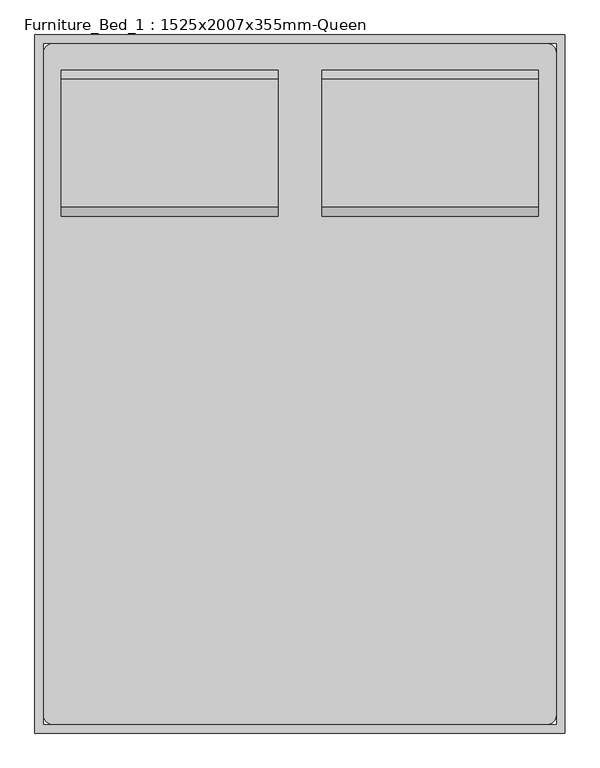
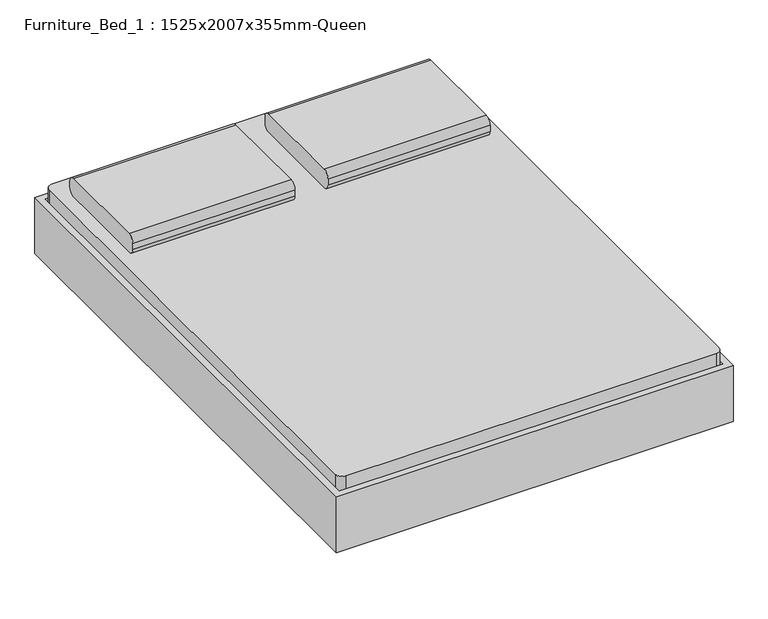
"""IFC4 building model written with IfcOpenShell, lengths in millimetres: furniture geometry, Furniture_Bed_1 : 1525x2007x355mm-Queen."""

from ifc_helpers import new_model, si_unit, point, frame, frame_2d, origin, place, context, project, spatial, polyline, circle_curve, trimmed, segment, composite_curve, outline, extrude, source, transform, mapped, element, save
from ifc_brep_helpers import plane_surface, cylinder_surface, revolved_surface, advanced_brep


def furniture_bed_1_1525x2007x355mm_queen_b7403446(model_context):
    return source(origin(), model_context, "Body", "SolidModel", [
        advanced_brep(
        [(-397.947541, -933.1295082, 196.85), (-397.947541, -933.1295082, 177.8), (-397.947541, -1009.3295082, 177.8), (-397.947541, -1009.3295082, 196.85), (-335.0113525, -933.1295082, 196.85), (-347.147541, -933.1295082, 177.8), (-347.147541, -1009.3295082, 177.8), (-335.0113525, -1009.3295082, 196.85), (-253.8115092, -933.1295082, 22.716374), (-271.0766725, -933.1295082, 14.6654962), (-271.0766725, -1009.3295082, 14.6654962), (-253.8115092, -1009.3295082, 22.716374), (-248.0564547, -933.1295082, 0.0), (-248.0564547, -933.1295082, 19.05), (-248.0564547, -1009.3295082, 0.0), (-248.0564547, -1009.3295082, 19.05), (-169.4439489, -933.1295082, 19.05), (-169.4439489, -933.1295082, 0.0), (-169.4439489, -1009.3295082, 0.0), (-169.4439489, -1009.3295082, 19.05), (-156.7439489, -933.1295082, 3.4029547), (-166.2689489, -933.1295082, 19.9007387), (-156.7439489, -1009.3295082, 3.4029547), (-166.2689489, -1009.3295082, 19.9007387), (-101.7513357, -933.1295082, 57.15), (-96.6469036, -933.1295082, 38.1), (-96.6469036, -1009.3295082, 38.1), (-101.7513357, -1009.3295082, 57.15), (780.0562537, -933.1295082, 57.15), (774.9518216, -933.1295082, 38.1), (774.9518216, -1009.3295082, 38.1), (780.0562537, -1009.3295082, 57.15), (844.5738669, -933.1295082, 19.9007387), (835.0488669, -933.1295082, 3.4029547), (835.0488669, -1009.3295082, 3.4029547), (844.5738669, -1009.3295082, 19.9007387), (847.7488669, -933.1295082, 0.0), (847.7488669, -933.1295082, 19.05), (847.7488669, -1009.3295082, 0.0), (847.7488669, -1009.3295082, 19.05), (926.3613728, -933.1295082, 19.05), (926.3613728, -933.1295082, 0.0), (926.3613728, -1009.3295082, 0.0), (926.3613728, -1009.3295082, 19.05), (949.3815906, -933.1295082, 14.6654962), (932.1164272, -933.1295082, 22.716374), (949.3815906, -1009.3295082, 14.6654962), (932.1164272, -1009.3295082, 22.716374), (1013.3162705, -933.1295082, 196.85), (1025.452459, -933.1295082, 177.8), (1025.452459, -1009.3295082, 177.8), (1013.3162705, -1009.3295082, 196.85), (1076.252459, -933.1295082, 196.85), (1076.252459, -1009.3295082, 196.85), (1076.252459, -1009.3295082, 177.8), (1076.252459, -933.1295082, 177.8)],
        [
            (0, 1),
            (1, 2),
            (2, 3),
            (3, 0),
            (0, 4),
            (4, 5),
            (5, 1),
            (5, 6),
            (6, 2),
            (6, 7),
            (7, 3),
            (7, 4),
            (4, 8),
            (8, 9),
            (9, 5),
            (9, 10),
            (10, 6),
            (10, 11),
            (11, 7),
            (11, 8),
            (12, 9, circle_curve(frame((-248.0564547, -933.1295082, 25.4), z_axis=(0.0, 1.0, 0.0), x_axis=(-0.9063077870366627, 0.0, -0.42261826174067213)), 25.4)),
            (8, 13, circle_curve(frame((-248.0564547, -933.1295082, 25.4), z_axis=(0.0, -1.0, 0.0), x_axis=(-0.9063077870366627, 0.0, -0.42261826174067213)), 6.35)),
            (13, 12),
            (14, 10, circle_curve(frame((-248.0564547, -1009.3295082, 25.4), z_axis=(0.0, 1.0, 0.0), x_axis=(-0.9063077870366627, 0.0, -0.42261826174067213)), 25.4)),
            (12, 14),
            (15, 11, circle_curve(frame((-248.0564547, -1009.3295082, 25.4), z_axis=(0.0, 1.0, 0.0), x_axis=(-0.9063077870366627, 0.0, -0.42261826174067213)), 6.35)),
            (14, 15),
            (15, 13),
            (13, 16),
            (16, 17),
            (17, 12),
            (17, 18),
            (18, 14),
            (18, 19),
            (19, 15),
            (19, 16),
            (20, 17, circle_curve(frame((-169.4439489, -933.1295082, 25.4), z_axis=(0.0, 1.0, 0.0), x_axis=(0.0, 0.0, -1.0)), 25.4)),
            (16, 21, circle_curve(frame((-169.4439489, -933.1295082, 25.4), z_axis=(0.0, -1.0, 0.0), x_axis=(0.0, 0.0, -1.0)), 6.35)),
            (21, 20),
            (22, 18, circle_curve(frame((-169.4439489, -1009.3295082, 25.4), z_axis=(0.0, 1.0, 0.0), x_axis=(0.0, 0.0, -1.0)), 25.4)),
            (20, 22),
            (23, 19, circle_curve(frame((-169.4439489, -1009.3295082, 25.4), z_axis=(0.0, 1.0, 0.0), x_axis=(0.0, 0.0, -1.0)), 6.35)),
            (22, 23),
            (23, 21),
            (21, 24),
            (24, 25),
            (25, 20),
            (25, 26),
            (26, 22),
            (26, 27),
            (27, 23),
            (27, 24),
            (24, 28),
            (28, 29),
            (29, 25),
            (29, 30),
            (30, 26),
            (30, 31),
            (31, 27),
            (31, 28),
            (28, 32),
            (32, 33),
            (33, 29),
            (33, 34),
            (34, 30),
            (34, 35),
            (35, 31),
            (35, 32),
            (36, 33, circle_curve(frame((847.7488669, -933.1295082, 25.4), z_axis=(0.0, 1.0, 0.0), x_axis=(-0.5000000000000486, 0.0, -0.8660254037844105)), 25.4)),
            (32, 37, circle_curve(frame((847.7488669, -933.1295082, 25.4), z_axis=(0.0, -1.0, 0.0), x_axis=(-0.5000000000000486, 0.0, -0.8660254037844105)), 6.35)),
            (37, 36),
            (38, 34, circle_curve(frame((847.7488669, -1009.3295082, 25.4), z_axis=(0.0, 1.0, 0.0), x_axis=(-0.5000000000000486, 0.0, -0.8660254037844105)), 25.4)),
            (36, 38),
            (39, 35, circle_curve(frame((847.7488669, -1009.3295082, 25.4), z_axis=(0.0, 1.0, 0.0), x_axis=(-0.5000000000000486, 0.0, -0.8660254037844105)), 6.35)),
            (38, 39),
            (39, 37),
            (37, 40),
            (40, 41),
            (41, 36),
            (41, 42),
            (42, 38),
            (42, 43),
            (43, 39),
            (43, 40),
            (44, 41, circle_curve(frame((926.3613728, -933.1295082, 25.4), z_axis=(0.0, 1.0, 0.0), x_axis=(0.0, 0.0, -1.0)), 25.4)),
            (40, 45, circle_curve(frame((926.3613728, -933.1295082, 25.4), z_axis=(0.0, -1.0, 0.0), x_axis=(0.0, 0.0, -1.0)), 6.35)),
            (45, 44),
            (46, 42, circle_curve(frame((926.3613728, -1009.3295082, 25.4), z_axis=(0.0, 1.0, 0.0), x_axis=(0.0, 0.0, -1.0)), 25.4)),
            (44, 46),
            (47, 43, circle_curve(frame((926.3613728, -1009.3295082, 25.4), z_axis=(0.0, 1.0, 0.0), x_axis=(0.0, 0.0, -1.0)), 6.35)),
            (46, 47),
            (47, 45),
            (45, 48),
            (48, 49),
            (49, 44),
            (49, 50),
            (50, 46),
            (50, 51),
            (51, 47),
            (51, 48),
            (52, 53),
            (53, 54),
            (54, 55),
            (55, 52),
            (48, 52),
            (55, 49),
            (54, 50),
            (53, 51),
        ],
        [
            plane_surface(frame((-397.947541, -1237.9295082, -127.5947323), z_axis=(-1.0, 0.0, 0.0), x_axis=(0.0, 1.0, 0.0))),
            plane_surface(frame((-397.947541, -933.1295082, 196.85), z_axis=(0.0, 1.0, 0.0), x_axis=(1.0, 0.0, 0.0))),
            plane_surface(frame((-397.947541, -933.1295082, 177.8), z_axis=(0.0, 0.0, -1.0), x_axis=(1.0, 0.0, 0.0))),
            plane_surface(frame((-397.947541, -1009.3295082, 177.8), z_axis=(0.0, -1.0, 0.0), x_axis=(1.0, 0.0, 0.0))),
            plane_surface(frame((-397.947541, -1009.3295082, 196.85), z_axis=(0.0, 0.0, 1.0), x_axis=(1.0, 0.0, 0.0))),
            plane_surface(frame((-335.0113525, -933.1295082, 196.85), z_axis=(0.0, 1.0000000000000002, 0.0), x_axis=(0.4226182617406718, 0.0, -0.9063077870366629))),
            plane_surface(frame((-347.147541, -933.1295082, 177.8), z_axis=(-0.906307787036663, 0.0, -0.4226182617406716), x_axis=(0.4226182617406716, 0.0, -0.906307787036663))),
            plane_surface(frame((-347.147541, -1009.3295082, 177.8), z_axis=(0.0, -1.0000000000000002, 0.0), x_axis=(0.4226182617406718, 0.0, -0.9063077870366629))),
            plane_surface(frame((-335.0113525, -1009.3295082, 196.85), z_axis=(0.9063077870366628, 0.0, 0.42261826174067196), x_axis=(0.42261826174067196, 0.0, -0.9063077870366628))),
            plane_surface(frame((-248.0564547, -933.1295082, 25.4), z_axis=(0.0, 1.0, 0.0), x_axis=(-0.9063077870366627, 0.0, -0.42261826174067213))),
            cylinder_surface(frame((-248.0564547, -1237.9295082, 25.4), z_axis=(0.0, -1.0, 0.0), x_axis=(-0.9063077870366627, 0.0, -0.42261826174067213)), 25.4),
            plane_surface(frame((-248.0564547, -1009.3295082, 25.4), z_axis=(0.0, -1.0, 0.0), x_axis=(-0.9063077870366627, 0.0, -0.42261826174067213))),
            revolved_surface(polyline([(-253.81150914768278, -1009.3295082, 22.716374037946732), (-253.81150914768278, -933.1295082, 22.716374037946732)]), (-248.0564547, -1237.9295082, 25.4), (0.0, -1.0, 0.0)),
            plane_surface(frame((-248.0564547, -933.1295082, 19.05), z_axis=(0.0, 1.0, 0.0), x_axis=(1.0, 0.0, 0.0))),
            plane_surface(frame((-248.0564547, -933.1295082, 0.0), z_axis=(0.0, 0.0, -1.0), x_axis=(1.0, 0.0, 0.0))),
            plane_surface(frame((-248.0564547, -1009.3295082, 0.0), z_axis=(0.0, -1.0, 0.0), x_axis=(1.0, 0.0, 0.0))),
            plane_surface(frame((-248.0564547, -1009.3295082, 19.05), z_axis=(0.0, 0.0, 1.0), x_axis=(1.0, 0.0, 0.0))),
            plane_surface(frame((-169.4439489, -933.1295082, 25.4), z_axis=(0.0, 1.0, 0.0), x_axis=(0.0, 0.0, -1.0))),
            cylinder_surface(frame((-169.4439489, -1237.9295082, 25.4), z_axis=(0.0, -1.0, 0.0), x_axis=(0.0, 0.0, -1.0)), 25.4),
            plane_surface(frame((-169.4439489, -1009.3295082, 25.4), z_axis=(0.0, -1.0, 0.0), x_axis=(0.0, 0.0, -1.0))),
            revolved_surface(polyline([(-169.4439489, -1009.3295082, 19.049999999999997), (-169.4439489, -933.1295082, 19.049999999999997)]), (-169.4439489, -1237.9295082, 25.4), (0.0, -1.0, 0.0)),
            plane_surface(frame((-166.2689489, -933.1295082, 19.9007387), z_axis=(0.0, 1.0, 0.0), x_axis=(0.8660254037844786, 0.0, 0.4999999999999309))),
            plane_surface(frame((-156.7439489, -933.1295082, 3.4029547), z_axis=(0.4999999999999315, 0.0, -0.8660254037844782), x_axis=(0.8660254037844782, 0.0, 0.4999999999999315))),
            plane_surface(frame((-156.7439489, -1009.3295082, 3.4029547), z_axis=(0.0, -1.0, 0.0), x_axis=(0.8660254037844788, 0.0, 0.49999999999993044))),
            plane_surface(frame((-166.2689489, -1009.3295082, 19.9007387), z_axis=(-0.4999999999999304, 0.0, 0.8660254037844789), x_axis=(0.8660254037844789, 0.0, 0.4999999999999304))),
            plane_surface(frame((-101.7513357, -933.1295082, 57.15), z_axis=(0.0, 1.0, 0.0), x_axis=(1.0, 0.0, 0.0))),
            plane_surface(frame((-96.6469036, -933.1295082, 38.1), z_axis=(0.0, 0.0, -1.0), x_axis=(1.0, 0.0, 0.0))),
            plane_surface(frame((-96.6469036, -1009.3295082, 38.1), z_axis=(0.0, -1.0, 0.0), x_axis=(1.0, 0.0, 0.0))),
            plane_surface(frame((-101.7513357, -1009.3295082, 57.15), z_axis=(0.0, 0.0, 1.0), x_axis=(1.0, 0.0, 0.0))),
            plane_surface(frame((780.0562537, -933.1295082, 57.15), z_axis=(0.0, 1.0, 0.0), x_axis=(0.866025403784412, 0.0, -0.5000000000000463))),
            plane_surface(frame((774.9518216, -933.1295082, 38.1), z_axis=(-0.500000000000047, 0.0, -0.8660254037844116), x_axis=(0.8660254037844116, 0.0, -0.500000000000047))),
            plane_surface(frame((774.9518216, -1009.3295082, 38.1), z_axis=(0.0, -1.0, 0.0), x_axis=(0.866025403784411, 0.0, -0.5000000000000481))),
            plane_surface(frame((780.0562537, -1009.3295082, 57.15), z_axis=(0.5000000000000471, 0.0, 0.8660254037844115), x_axis=(0.8660254037844115, 0.0, -0.5000000000000471))),
            plane_surface(frame((847.7488669, -933.1295082, 25.4), z_axis=(0.0, 1.0000000000000002, 0.0), x_axis=(-0.5000000000000487, 0.0, -0.8660254037844106))),
            cylinder_surface(frame((847.7488669, -1237.9295082, 25.4), z_axis=(0.0, -1.0, 0.0), x_axis=(-0.5000000000000486, 0.0, -0.8660254037844105)), 25.4),
            plane_surface(frame((847.7488669, -1009.3295082, 25.4), z_axis=(0.0, -1.0000000000000002, 0.0), x_axis=(-0.5000000000000487, 0.0, -0.8660254037844106))),
            revolved_surface(polyline([(844.5738668999998, -1009.3295082, 19.900738685968992), (844.5738668999998, -933.1295082, 19.900738685968992)]), (847.7488669, -1237.9295082, 25.4), (0.0, -1.0, 0.0)),
            plane_surface(frame((847.7488669, -933.1295082, 19.05), z_axis=(0.0, 1.0, 0.0), x_axis=(1.0, 0.0, 0.0))),
            plane_surface(frame((847.7488669, -933.1295082, 0.0), z_axis=(0.0, 0.0, -1.0), x_axis=(1.0, 0.0, 0.0))),
            plane_surface(frame((847.7488669, -1009.3295082, 0.0), z_axis=(0.0, -1.0, 0.0), x_axis=(1.0, 0.0, 0.0))),
            plane_surface(frame((847.7488669, -1009.3295082, 19.05), z_axis=(0.0, 0.0, 1.0), x_axis=(1.0, 0.0, 0.0))),
            plane_surface(frame((926.3613728, -933.1295082, 25.4), z_axis=(0.0, 1.0, 0.0), x_axis=(0.0, 0.0, -1.0))),
            cylinder_surface(frame((926.3613728, -1237.9295082, 25.4), z_axis=(0.0, -1.0, 0.0), x_axis=(0.0, 0.0, -1.0)), 25.4),
            plane_surface(frame((926.3613728, -1009.3295082, 25.4), z_axis=(0.0, -1.0, 0.0), x_axis=(0.0, 0.0, -1.0))),
            revolved_surface(polyline([(926.3613728, -1009.3295082, 19.049999999999997), (926.3613728, -933.1295082, 19.049999999999997)]), (926.3613728, -1237.9295082, 25.4), (0.0, -1.0, 0.0)),
            plane_surface(frame((932.1164272, -933.1295082, 22.716374), z_axis=(0.0, 1.0, 0.0), x_axis=(0.4226182617405395, 0.0, 0.9063077870367245))),
            plane_surface(frame((949.3815906, -933.1295082, 14.6654962), z_axis=(0.9063077870367247, 0.0, -0.4226182617405394), x_axis=(0.4226182617405394, 0.0, 0.9063077870367247))),
            plane_surface(frame((949.3815906, -1009.3295082, 14.6654962), z_axis=(0.0, -1.0, 0.0), x_axis=(0.4226182617405393, 0.0, 0.9063077870367247))),
            plane_surface(frame((932.1164272, -1009.3295082, 22.716374), z_axis=(-0.9063077870367245, 0.0, 0.42261826174053974), x_axis=(0.42261826174053974, 0.0, 0.9063077870367245))),
            plane_surface(frame((1076.252459, -1237.9295082, -127.5947323), z_axis=(1.0, 0.0, 0.0), x_axis=(0.0, 1.0, 0.0))),
            plane_surface(frame((1013.3162705, -933.1295082, 196.85), z_axis=(0.0, 1.0, 0.0), x_axis=(1.0, 0.0, 0.0))),
            plane_surface(frame((1025.452459, -933.1295082, 177.8), z_axis=(0.0, 0.0, -1.0), x_axis=(1.0, 0.0, 0.0))),
            plane_surface(frame((1025.452459, -1009.3295082, 177.8), z_axis=(0.0, -1.0, 0.0), x_axis=(1.0, 0.0, 0.0))),
            plane_surface(frame((1013.3162705, -1009.3295082, 196.85), z_axis=(0.0, 0.0, 1.0), x_axis=(1.0, 0.0, 0.0))),
        ],
        [
            (0, [[1, 2, 3, 4]]),
            (1, [[-1, 5, 6, 7]]),
            (2, [[-2, -7, 8, 9]]),
            (3, [[-3, -9, 10, 11]]),
            (4, [[-4, -11, 12, -5]]),
            (5, [[-6, 13, 14, 15]]),
            (6, [[-8, -15, 16, 17]]),
            (7, [[-10, -17, 18, 19]]),
            (8, [[-12, -19, 20, -13]]),
            (9, [[21, -14, 22, 23]]),
            (10, [[24, -16, -21, 25]]),
            (11, [[26, -18, -24, 27]]),
            (12, [[-22, -20, -26, 28]]),
            (13, [[-23, 29, 30, 31]]),
            (14, [[-25, -31, 32, 33]]),
            (15, [[-27, -33, 34, 35]]),
            (16, [[-28, -35, 36, -29]]),
            (17, [[37, -30, 38, 39]]),
            (18, [[40, -32, -37, 41]]),
            (19, [[42, -34, -40, 43]]),
            (20, [[-38, -36, -42, 44]]),
            (21, [[-39, 45, 46, 47]]),
            (22, [[-41, -47, 48, 49]]),
            (23, [[-43, -49, 50, 51]]),
            (24, [[-44, -51, 52, -45]]),
            (25, [[-46, 53, 54, 55]]),
            (26, [[-48, -55, 56, 57]]),
            (27, [[-50, -57, 58, 59]]),
            (28, [[-52, -59, 60, -53]]),
            (29, [[-54, 61, 62, 63]]),
            (30, [[-56, -63, 64, 65]]),
            (31, [[-58, -65, 66, 67]]),
            (32, [[-60, -67, 68, -61]]),
            (33, [[69, -62, 70, 71]]),
            (34, [[72, -64, -69, 73]]),
            (35, [[74, -66, -72, 75]]),
            (36, [[-70, -68, -74, 76]]),
            (37, [[-71, 77, 78, 79]]),
            (38, [[-73, -79, 80, 81]]),
            (39, [[-75, -81, 82, 83]]),
            (40, [[-76, -83, 84, -77]]),
            (41, [[85, -78, 86, 87]]),
            (42, [[88, -80, -85, 89]]),
            (43, [[90, -82, -88, 91]]),
            (44, [[-86, -84, -90, 92]]),
            (45, [[-87, 93, 94, 95]]),
            (46, [[-89, -95, 96, 97]]),
            (47, [[-91, -97, 98, 99]]),
            (48, [[-92, -99, 100, -93]]),
            (49, [[101, 102, 103, 104]]),
            (50, [[-94, 105, -104, 106]]),
            (51, [[-96, -106, -103, 107]]),
            (52, [[-98, -107, -102, 108]]),
            (53, [[-100, -108, -101, -105]]),
        ],
    ),
        extrude(outline(composite_curve([segment(polyline([(-372.547541, 743.6704918), (1050.852459, 743.6704918)]), True, "CONTINUOUS"), segment(trimmed(circle_curve(frame_2d((1050.852459, 718.2704918)), 25.4), [point((1050.852459, 743.6704918))], [point((1076.252459, 718.2704918))], False, "CARTESIAN"), True, "CONTINUOUS"), segment(polyline([(1076.252459, 718.2704918), (1076.252459, -1187.1295082)]), True, "CONTINUOUS"), segment(trimmed(circle_curve(frame_2d((1050.852459, -1187.1295082)), 25.4), [point((1076.252459, -1187.1295082))], [point((1050.852459, -1212.5295082))], False, "CARTESIAN"), True, "CONTINUOUS"), segment(polyline([(1050.852459, -1212.5295082), (-372.547541, -1212.5295082)]), True, "CONTINUOUS"), segment(trimmed(circle_curve(frame_2d((-372.547541, -1187.1295082)), 25.4), [point((-372.547541, -1212.5295082))], [point((-397.947541, -1187.1295082))], False, "CARTESIAN"), True, "CONTINUOUS"), segment(polyline([(-397.947541, -1187.1295082), (-397.947541, 718.2704918)]), True, "CONTINUOUS"), segment(trimmed(circle_curve(frame_2d((-372.547541, 718.2704918)), 25.4), [point((-397.947541, 718.2704918))], [point((-372.547541, 743.6704918))], False, "CARTESIAN"), True, "CONTINUOUS")], self_intersect=False)), frame((0.0, 0.0, 203.2), z_axis=(0.0, 0.0, 1.0), x_axis=(1.0, 0.0, 0.0)), (0.0, 0.0, 1.0), 203.2),
        advanced_brep(
        [(-397.6231784, 515.0704918, 177.8), (-397.6231784, 438.8704918, 177.8), (-397.6231784, 438.8704918, 196.85), (-397.6231784, 515.0704918, 196.85), (-346.8231784, 515.0704918, 177.8), (-346.8231784, 438.8704918, 177.8), (-334.6869899, 438.8704918, 196.85), (-334.6869899, 515.0704918, 196.85), (-270.7523099, 515.0704918, 14.6654962), (-270.7523099, 438.8704918, 14.6654962), (-253.4871466, 438.8704918, 22.716374), (-253.4871466, 515.0704918, 22.716374), (-247.7320921, 438.8704918, 0.0), (-247.7320921, 515.0704918, 0.0), (-247.7320921, 438.8704918, 19.05), (-247.7320921, 515.0704918, 19.05), (-169.1195862, 515.0704918, 0.0), (-169.1195862, 438.8704918, 0.0), (-169.1195862, 438.8704918, 19.05), (-169.1195862, 515.0704918, 19.05), (-156.4195862, 438.8704918, 3.4029547), (-156.4195862, 515.0704918, 3.4029547), (-165.9445862, 438.8704918, 19.9007387), (-165.9445862, 515.0704918, 19.9007387), (-96.322541, 515.0704918, 38.1), (-96.322541, 438.8704918, 38.1), (-101.4269731, 438.8704918, 57.15), (-101.4269731, 515.0704918, 57.15), (774.9518216, 515.0704918, 38.1), (774.9518216, 438.8704918, 38.1), (780.0562537, 438.8704918, 57.15), (780.0562537, 515.0704918, 57.15), (835.0488669, 515.0704918, 3.4029547), (835.0488669, 438.8704918, 3.4029547), (844.5738669, 438.8704918, 19.9007387), (844.5738669, 515.0704918, 19.9007387), (847.7488669, 438.8704918, 0.0), (847.7488669, 515.0704918, 0.0), (847.7488669, 438.8704918, 19.05), (847.7488669, 515.0704918, 19.05), (926.3613728, 515.0704918, 0.0), (926.3613728, 438.8704918, 0.0), (926.3613728, 438.8704918, 19.05), (926.3613728, 515.0704918, 19.05), (949.3815906, 438.8704918, 14.6654962), (949.3815906, 515.0704918, 14.6654962), (932.1164272, 438.8704918, 22.716374), (932.1164272, 515.0704918, 22.716374), (1025.452459, 515.0704918, 177.8), (1025.452459, 438.8704918, 177.8), (1013.3162705, 438.8704918, 196.85), (1013.3162705, 515.0704918, 196.85), (1076.252459, 515.0704918, 177.8), (1076.252459, 515.0704918, 196.85), (1076.252459, 438.8704918, 196.85), (1076.252459, 438.8704918, 177.8)],
        [
            (0, 1),
            (1, 2),
            (2, 3),
            (3, 0),
            (0, 4),
            (4, 5),
            (5, 1),
            (5, 6),
            (6, 2),
            (6, 7),
            (7, 3),
            (7, 4),
            (4, 8),
            (8, 9),
            (9, 5),
            (9, 10),
            (10, 6),
            (10, 11),
            (11, 7),
            (11, 8),
            (12, 9, circle_curve(frame((-247.7320921, 438.8704918, 25.4), z_axis=(0.0, 1.0, 0.0), x_axis=(-0.906307787036649, 0.0, -0.4226182617407015)), 25.4)),
            (8, 13, circle_curve(frame((-247.7320921, 515.0704918, 25.4), z_axis=(0.0, -1.0, 0.0), x_axis=(-0.906307787036649, 0.0, -0.4226182617407015)), 25.4)),
            (13, 12),
            (14, 10, circle_curve(frame((-247.7320921, 438.8704918, 25.4), z_axis=(0.0, 1.0, 0.0), x_axis=(-0.906307787036649, 0.0, -0.4226182617407015)), 6.35)),
            (12, 14),
            (15, 11, circle_curve(frame((-247.7320921, 515.0704918, 25.4), z_axis=(0.0, 1.0, 0.0), x_axis=(-0.906307787036649, 0.0, -0.4226182617407015)), 6.35)),
            (14, 15),
            (15, 13),
            (13, 16),
            (16, 17),
            (17, 12),
            (17, 18),
            (18, 14),
            (18, 19),
            (19, 15),
            (19, 16),
            (20, 17, circle_curve(frame((-169.1195862, 438.8704918, 25.4), z_axis=(0.0, 1.0, 0.0), x_axis=(0.0, 0.0, -1.0)), 25.4)),
            (16, 21, circle_curve(frame((-169.1195862, 515.0704918, 25.4), z_axis=(0.0, -1.0, 0.0), x_axis=(0.0, 0.0, -1.0)), 25.4)),
            (21, 20),
            (22, 18, circle_curve(frame((-169.1195862, 438.8704918, 25.4), z_axis=(0.0, 1.0, 0.0), x_axis=(0.0, 0.0, -1.0)), 6.35)),
            (20, 22),
            (23, 19, circle_curve(frame((-169.1195862, 515.0704918, 25.4), z_axis=(0.0, 1.0, 0.0), x_axis=(0.0, 0.0, -1.0)), 6.35)),
            (22, 23),
            (23, 21),
            (21, 24),
            (24, 25),
            (25, 20),
            (25, 26),
            (26, 22),
            (26, 27),
            (27, 23),
            (27, 24),
            (24, 28),
            (28, 29),
            (29, 25),
            (29, 30),
            (30, 26),
            (30, 31),
            (31, 27),
            (31, 28),
            (28, 32),
            (32, 33),
            (33, 29),
            (33, 34),
            (34, 30),
            (34, 35),
            (35, 31),
            (35, 32),
            (36, 33, circle_curve(frame((847.7488669, 438.8704918, 25.4), z_axis=(0.0, 1.0, 0.0), x_axis=(-0.5000000000000444, 0.0, -0.866025403784413)), 25.4)),
            (32, 37, circle_curve(frame((847.7488669, 515.0704918, 25.4), z_axis=(0.0, -1.0, 0.0), x_axis=(-0.5000000000000444, 0.0, -0.866025403784413)), 25.4)),
            (37, 36),
            (38, 34, circle_curve(frame((847.7488669, 438.8704918, 25.4), z_axis=(0.0, 1.0, 0.0), x_axis=(-0.5000000000000444, 0.0, -0.866025403784413)), 6.35)),
            (36, 38),
            (39, 35, circle_curve(frame((847.7488669, 515.0704918, 25.4), z_axis=(0.0, 1.0, 0.0), x_axis=(-0.5000000000000444, 0.0, -0.866025403784413)), 6.35)),
            (38, 39),
            (39, 37),
            (37, 40),
            (40, 41),
            (41, 36),
            (41, 42),
            (42, 38),
            (42, 43),
            (43, 39),
            (43, 40),
            (44, 41, circle_curve(frame((926.3613728, 438.8704918, 25.4), z_axis=(0.0, 1.0, 0.0), x_axis=(0.0, 0.0, -1.0)), 25.4)),
            (40, 45, circle_curve(frame((926.3613728, 515.0704918, 25.4), z_axis=(0.0, -1.0, 0.0), x_axis=(0.0, 0.0, -1.0)), 25.4)),
            (45, 44),
            (46, 42, circle_curve(frame((926.3613728, 438.8704918, 25.4), z_axis=(0.0, 1.0, 0.0), x_axis=(0.0, 0.0, -1.0)), 6.35)),
            (44, 46),
            (47, 43, circle_curve(frame((926.3613728, 515.0704918, 25.4), z_axis=(0.0, 1.0, 0.0), x_axis=(0.0, 0.0, -1.0)), 6.35)),
            (46, 47),
            (47, 45),
            (45, 48),
            (48, 49),
            (49, 44),
            (49, 50),
            (50, 46),
            (50, 51),
            (51, 47),
            (51, 48),
            (52, 53),
            (53, 54),
            (54, 55),
            (55, 52),
            (48, 52),
            (55, 49),
            (54, 50),
            (53, 51),
        ],
        [
            plane_surface(frame((-397.6231784, 769.0704918, -152.9490627), z_axis=(-1.0, 0.0, 0.0), x_axis=(0.0, 1.0, 0.0))),
            plane_surface(frame((-397.6231784, 515.0704918, 177.8), z_axis=(0.0, 0.0, -1.0), x_axis=(1.0, 0.0, 0.0))),
            plane_surface(frame((-397.6231784, 438.8704918, 177.8), z_axis=(0.0, -1.0, 0.0), x_axis=(1.0, 0.0, 0.0))),
            plane_surface(frame((-397.6231784, 438.8704918, 196.85), z_axis=(0.0, 0.0, 1.0), x_axis=(1.0, 0.0, 0.0))),
            plane_surface(frame((-397.6231784, 515.0704918, 196.85), z_axis=(0.0, 1.0, 0.0), x_axis=(1.0, 0.0, 0.0))),
            plane_surface(frame((-346.8231784, 515.0704918, 177.8), z_axis=(-0.9063077870366485, 0.0, -0.4226182617407029), x_axis=(0.4226182617407029, 0.0, -0.9063077870366485))),
            plane_surface(frame((-346.8231784, 438.8704918, 177.8), z_axis=(0.0, -1.0, 0.0), x_axis=(0.42261826174070266, 0.0, -0.9063077870366485))),
            plane_surface(frame((-334.6869899, 438.8704918, 196.85), z_axis=(0.9063077870366486, 0.0, 0.4226182617407026), x_axis=(0.4226182617407026, 0.0, -0.9063077870366486))),
            plane_surface(frame((-334.6869899, 515.0704918, 196.85), z_axis=(0.0, 1.0, 0.0), x_axis=(0.42261826174070266, 0.0, -0.9063077870366485))),
            cylinder_surface(frame((-247.7320921, 769.0704918, 25.4), z_axis=(0.0, -1.0, 0.0), x_axis=(-0.906307787036649, 0.0, -0.4226182617407015)), 25.4),
            plane_surface(frame((-247.7320921, 438.8704918, 25.4), z_axis=(0.0, -1.0, 0.0), x_axis=(-0.906307787036649, 0.0, -0.4226182617407015))),
            revolved_surface(polyline([(-253.4871465476827, 438.8704918, 22.716374037946544), (-253.4871465476827, 515.0704918, 22.716374037946544)]), (-247.7320921, 769.0704918, 25.4), (0.0, -1.0, 0.0)),
            plane_surface(frame((-247.7320921, 515.0704918, 25.4), z_axis=(0.0, 1.0, 0.0), x_axis=(-0.906307787036649, 0.0, -0.4226182617407015))),
            plane_surface(frame((-247.7320921, 515.0704918, 0.0), z_axis=(0.0, 0.0, -1.0), x_axis=(1.0, 0.0, 0.0))),
            plane_surface(frame((-247.7320921, 438.8704918, 0.0), z_axis=(0.0, -1.0, 0.0), x_axis=(1.0, 0.0, 0.0))),
            plane_surface(frame((-247.7320921, 438.8704918, 19.05), z_axis=(0.0, 0.0, 1.0), x_axis=(1.0, 0.0, 0.0))),
            plane_surface(frame((-247.7320921, 515.0704918, 19.05), z_axis=(0.0, 1.0, 0.0), x_axis=(1.0, 0.0, 0.0))),
            cylinder_surface(frame((-169.1195862, 769.0704918, 25.4), z_axis=(0.0, -1.0, 0.0), x_axis=(0.0, 0.0, -1.0)), 25.4),
            plane_surface(frame((-169.1195862, 438.8704918, 25.4), z_axis=(0.0, -1.0, 0.0), x_axis=(0.0, 0.0, -1.0))),
            revolved_surface(polyline([(-169.1195862, 438.8704918, 19.049999999999997), (-169.1195862, 515.0704918, 19.049999999999997)]), (-169.1195862, 769.0704918, 25.4), (0.0, -1.0, 0.0)),
            plane_surface(frame((-169.1195862, 515.0704918, 25.4), z_axis=(0.0, 1.0, 0.0), x_axis=(0.0, 0.0, -1.0))),
            plane_surface(frame((-156.4195862, 515.0704918, 3.4029547), z_axis=(0.49999999999987826, 0.0, -0.866025403784509), x_axis=(0.866025403784509, 0.0, 0.49999999999987826))),
            plane_surface(frame((-156.4195862, 438.8704918, 3.4029547), z_axis=(0.0, -1.0, 0.0), x_axis=(0.8660254037845093, 0.0, 0.4999999999998776))),
            plane_surface(frame((-165.9445862, 438.8704918, 19.9007387), z_axis=(-0.4999999999998785, 0.0, 0.8660254037845089), x_axis=(0.8660254037845089, 0.0, 0.4999999999998785))),
            plane_surface(frame((-165.9445862, 515.0704918, 19.9007387), z_axis=(0.0, 1.0, 0.0), x_axis=(0.866025403784509, 0.0, 0.49999999999987826))),
            plane_surface(frame((-96.322541, 515.0704918, 38.1), z_axis=(0.0, 0.0, -1.0), x_axis=(1.0, 0.0, 0.0))),
            plane_surface(frame((-96.322541, 438.8704918, 38.1), z_axis=(0.0, -1.0, 0.0), x_axis=(1.0, 0.0, 0.0))),
            plane_surface(frame((-101.4269731, 438.8704918, 57.15), z_axis=(0.0, 0.0, 1.0), x_axis=(1.0, 0.0, 0.0))),
            plane_surface(frame((-101.4269731, 515.0704918, 57.15), z_axis=(0.0, 1.0, 0.0), x_axis=(1.0, 0.0, 0.0))),
            plane_surface(frame((774.9518216, 515.0704918, 38.1), z_axis=(-0.5000000000000451, 0.0, -0.8660254037844127), x_axis=(0.8660254037844127, 0.0, -0.5000000000000451))),
            plane_surface(frame((774.9518216, 438.8704918, 38.1), z_axis=(0.0, -1.0, 0.0), x_axis=(0.866025403784413, 0.0, -0.5000000000000446))),
            plane_surface(frame((780.0562537, 438.8704918, 57.15), z_axis=(0.5000000000000449, 0.0, 0.8660254037844127), x_axis=(0.8660254037844127, 0.0, -0.5000000000000449))),
            plane_surface(frame((780.0562537, 515.0704918, 57.15), z_axis=(0.0, 1.0, 0.0), x_axis=(0.8660254037844125, 0.0, -0.5000000000000454))),
            cylinder_surface(frame((847.7488669, 769.0704918, 25.4), z_axis=(0.0, -1.0, 0.0), x_axis=(-0.5000000000000444, 0.0, -0.866025403784413)), 25.4),
            plane_surface(frame((847.7488669, 438.8704918, 25.4), z_axis=(0.0, -1.0000000000000002, 0.0), x_axis=(-0.5000000000000445, 0.0, -0.8660254037844131))),
            revolved_surface(polyline([(844.5738668999998, 438.8704918, 19.900738685968975), (844.5738668999998, 515.0704918, 19.900738685968975)]), (847.7488669, 769.0704918, 25.4), (0.0, -1.0, 0.0)),
            plane_surface(frame((847.7488669, 515.0704918, 25.4), z_axis=(0.0, 1.0000000000000002, 0.0), x_axis=(-0.5000000000000445, 0.0, -0.8660254037844131))),
            plane_surface(frame((847.7488669, 515.0704918, 0.0), z_axis=(0.0, 0.0, -1.0), x_axis=(1.0, 0.0, 0.0))),
            plane_surface(frame((847.7488669, 438.8704918, 0.0), z_axis=(0.0, -1.0, 0.0), x_axis=(1.0, 0.0, 0.0))),
            plane_surface(frame((847.7488669, 438.8704918, 19.05), z_axis=(0.0, 0.0, 1.0), x_axis=(1.0, 0.0, 0.0))),
            plane_surface(frame((847.7488669, 515.0704918, 19.05), z_axis=(0.0, 1.0, 0.0), x_axis=(1.0, 0.0, 0.0))),
            cylinder_surface(frame((926.3613728, 769.0704918, 25.4), z_axis=(0.0, -1.0, 0.0), x_axis=(0.0, 0.0, -1.0)), 25.4),
            plane_surface(frame((926.3613728, 438.8704918, 25.4), z_axis=(0.0, -1.0, 0.0), x_axis=(0.0, 0.0, -1.0))),
            revolved_surface(polyline([(926.3613728, 438.8704918, 19.049999999999997), (926.3613728, 515.0704918, 19.049999999999997)]), (926.3613728, 769.0704918, 25.4), (0.0, -1.0, 0.0)),
            plane_surface(frame((926.3613728, 515.0704918, 25.4), z_axis=(0.0, 1.0, 0.0), x_axis=(0.0, 0.0, -1.0))),
            plane_surface(frame((949.3815906, 515.0704918, 14.6654962), z_axis=(0.9063077870366802, 0.0, -0.4226182617406346), x_axis=(0.4226182617406346, 0.0, 0.9063077870366802))),
            plane_surface(frame((949.3815906, 438.8704918, 14.6654962), z_axis=(0.0, -1.0, 0.0), x_axis=(0.42261826174063377, 0.0, 0.9063077870366806))),
            plane_surface(frame((932.1164272, 438.8704918, 22.716374), z_axis=(-0.9063077870366807, 0.0, 0.4226182617406337), x_axis=(0.4226182617406337, 0.0, 0.9063077870366807))),
            plane_surface(frame((932.1164272, 515.0704918, 22.716374), z_axis=(0.0, 1.0, 0.0), x_axis=(0.4226182617406339, 0.0, 0.9063077870366806))),
            plane_surface(frame((1076.252459, 769.0704918, -152.9490627), z_axis=(1.0, 0.0, 0.0), x_axis=(0.0, 1.0, 0.0))),
            plane_surface(frame((1025.452459, 515.0704918, 177.8), z_axis=(0.0, 0.0, -1.0), x_axis=(1.0, 0.0, 0.0))),
            plane_surface(frame((1025.452459, 438.8704918, 177.8), z_axis=(0.0, -1.0, 0.0), x_axis=(1.0, 0.0, 0.0))),
            plane_surface(frame((1013.3162705, 438.8704918, 196.85), z_axis=(0.0, 0.0, 1.0), x_axis=(1.0, 0.0, 0.0))),
            plane_surface(frame((1013.3162705, 515.0704918, 196.85), z_axis=(0.0, 1.0, 0.0), x_axis=(1.0, 0.0, 0.0))),
        ],
        [
            (0, [[1, 2, 3, 4]]),
            (1, [[-1, 5, 6, 7]]),
            (2, [[-2, -7, 8, 9]]),
            (3, [[-3, -9, 10, 11]]),
            (4, [[-4, -11, 12, -5]]),
            (5, [[-6, 13, 14, 15]]),
            (6, [[-8, -15, 16, 17]]),
            (7, [[-10, -17, 18, 19]]),
            (8, [[-12, -19, 20, -13]]),
            (9, [[21, -14, 22, 23]]),
            (10, [[24, -16, -21, 25]]),
            (11, [[26, -18, -24, 27]]),
            (12, [[-22, -20, -26, 28]]),
            (13, [[-23, 29, 30, 31]]),
            (14, [[-25, -31, 32, 33]]),
            (15, [[-27, -33, 34, 35]]),
            (16, [[-28, -35, 36, -29]]),
            (17, [[37, -30, 38, 39]]),
            (18, [[40, -32, -37, 41]]),
            (19, [[42, -34, -40, 43]]),
            (20, [[-38, -36, -42, 44]]),
            (21, [[-39, 45, 46, 47]]),
            (22, [[-41, -47, 48, 49]]),
            (23, [[-43, -49, 50, 51]]),
            (24, [[-44, -51, 52, -45]]),
            (25, [[-46, 53, 54, 55]]),
            (26, [[-48, -55, 56, 57]]),
            (27, [[-50, -57, 58, 59]]),
            (28, [[-52, -59, 60, -53]]),
            (29, [[-54, 61, 62, 63]]),
            (30, [[-56, -63, 64, 65]]),
            (31, [[-58, -65, 66, 67]]),
            (32, [[-60, -67, 68, -61]]),
            (33, [[69, -62, 70, 71]]),
            (34, [[72, -64, -69, 73]]),
            (35, [[74, -66, -72, 75]]),
            (36, [[-70, -68, -74, 76]]),
            (37, [[-71, 77, 78, 79]]),
            (38, [[-73, -79, 80, 81]]),
            (39, [[-75, -81, 82, 83]]),
            (40, [[-76, -83, 84, -77]]),
            (41, [[85, -78, 86, 87]]),
            (42, [[88, -80, -85, 89]]),
            (43, [[90, -82, -88, 91]]),
            (44, [[-86, -84, -90, 92]]),
            (45, [[-87, 93, 94, 95]]),
            (46, [[-89, -95, 96, 97]]),
            (47, [[-91, -97, 98, 99]]),
            (48, [[-92, -99, 100, -93]]),
            (49, [[101, 102, 103, 104]]),
            (50, [[-94, 105, -104, 106]]),
            (51, [[-96, -106, -103, 107]]),
            (52, [[-98, -107, -102, 108]]),
            (53, [[-100, -108, -101, -105]]),
        ],
    ),
        extrude(outline(composite_curve([segment(polyline([(642.0704918, 406.4), (273.7704918, 406.4)]), True, "CONTINUOUS"), segment(trimmed(circle_curve(frame_2d((273.7704918, 431.8)), 25.4), [point((273.7704918, 406.4))], [point((248.3704918, 431.8))], False, "CARTESIAN"), True, "CONTINUOUS"), segment(polyline([(248.3704918, 431.8), (248.3704918, 457.2)]), True, "CONTINUOUS"), segment(trimmed(circle_curve(frame_2d((273.7704918, 457.2)), 25.4), [point((248.3704918, 457.2))], [point((273.7704918, 482.6))], False, "CARTESIAN"), True, "CONTINUOUS"), segment(polyline([(273.7704918, 482.6), (642.0704918, 482.6)]), True, "CONTINUOUS"), segment(trimmed(circle_curve(frame_2d((642.0704918, 457.2)), 25.4), [point((642.0704918, 482.6))], [point((667.4704918, 457.2))], False, "CARTESIAN"), True, "CONTINUOUS"), segment(polyline([(667.4704918, 457.2), (667.4704918, 431.8)]), True, "CONTINUOUS"), segment(trimmed(circle_curve(frame_2d((642.0704918, 431.8)), 25.4), [point((667.4704918, 431.8))], [point((642.0704918, 406.4))], False, "CARTESIAN"), True, "CONTINUOUS")], self_intersect=False)), frame((-347.147541, 0.0, 0.0), z_axis=(1.0, 0.0, 0.0), x_axis=(0.0, 1.0, 0.0)), (0.0, 0.0, 1.0), 622.8),
        extrude(outline(composite_curve([segment(polyline([(642.0704918, 406.4), (273.7704918, 406.4)]), True, "CONTINUOUS"), segment(trimmed(circle_curve(frame_2d((273.7704918, 431.8)), 25.4), [point((273.7704918, 406.4))], [point((248.3704918, 431.8))], False, "CARTESIAN"), True, "CONTINUOUS"), segment(polyline([(248.3704918, 431.8), (248.3704918, 457.2)]), True, "CONTINUOUS"), segment(trimmed(circle_curve(frame_2d((273.7704918, 457.2)), 25.4), [point((248.3704918, 457.2))], [point((273.7704918, 482.6))], False, "CARTESIAN"), True, "CONTINUOUS"), segment(polyline([(273.7704918, 482.6), (642.0704918, 482.6)]), True, "CONTINUOUS"), segment(trimmed(circle_curve(frame_2d((642.0704918, 457.2)), 25.4), [point((642.0704918, 482.6))], [point((667.4704918, 457.2))], False, "CARTESIAN"), True, "CONTINUOUS"), segment(polyline([(667.4704918, 457.2), (667.4704918, 431.8)]), True, "CONTINUOUS"), segment(trimmed(circle_curve(frame_2d((642.0704918, 431.8)), 25.4), [point((667.4704918, 431.8))], [point((642.0704918, 406.4))], False, "CARTESIAN"), True, "CONTINUOUS")], self_intersect=False)), frame((402.652459, 0.0, 0.0), z_axis=(1.0, 0.0, 0.0), x_axis=(0.0, 1.0, 0.0)), (0.0, 0.0, 1.0), 622.8),
        extrude(outline(polyline([(1101.652459, 769.0704918), (1101.652459, -1237.9295082), (-423.347541, -1237.9295082), (-423.347541, 769.0704918), (1101.652459, 769.0704918)]), holes=[polyline([(1076.252459, 743.6704918), (-397.947541, 743.6704918), (-397.947541, -1212.5295082), (1076.252459, -1212.5295082), (1076.252459, 743.6704918)])]), frame((0.0, 0.0, 127.0), z_axis=(0.0, 0.0, 1.0), x_axis=(1.0, 0.0, 0.0)), (0.0, 0.0, 1.0), 228.6),
    ])


if __name__ == "__main__":
    model = new_model("IFC4")
    model_context = context("Model", 3, world=origin())
    ifc_project = project(units=[si_unit("LENGTHUNIT", "METRE", prefix="MILLI")], contexts=[model_context])
    site = spatial("IfcSite", under=ifc_project)
    building = spatial("IfcBuilding", under=site)
    placement = place(None, origin())
    furniture_bed_1_1525x2007x355mm_queen_shape = furniture_bed_1_1525x2007x355mm_queen_b7403446(model_context)
    element("IfcFurniture", 1, ObjectType="Furniture_Bed_1 : 1525x2007x355mm-Queen", at=placement, inside=building, context=model_context, shape_type="MappedRepresentation", body=[
        mapped(furniture_bed_1_1525x2007x355mm_queen_shape, transform((0.0, 0.0, 0.0), x_axis=(1.0, 0.0, 0.0), y_axis=(0.0, 1.0, 0.0), z_axis=(0.0, 0.0, 1.0))),
    ])
    save(model, "model.ifc")

# Revit data of these elements
# Type "Furniture_Bed_1 : 1525x2007x355mm-Queen"
#   Keynote = "N"
#   Length = 6.584646 ft
#   Width = 5.003281 ft
#   Material Frame = Wood - Birch
#   Material Mattress = Textile - White
#   Default Elevation = 0
# Element 1 (IfcFurniture, "Furniture_Bed_1 : 1525x2007x355mm-Queen")
#   Materials on its faces: "Wood - Birch", "Textile - White"
# Materials
#   "Wood - Birch": class "Wood", colour RGB 224 178 126, transparency 0
#   "Textile - White": class "Fabric", colour RGB 247 247 239, transparency 0
